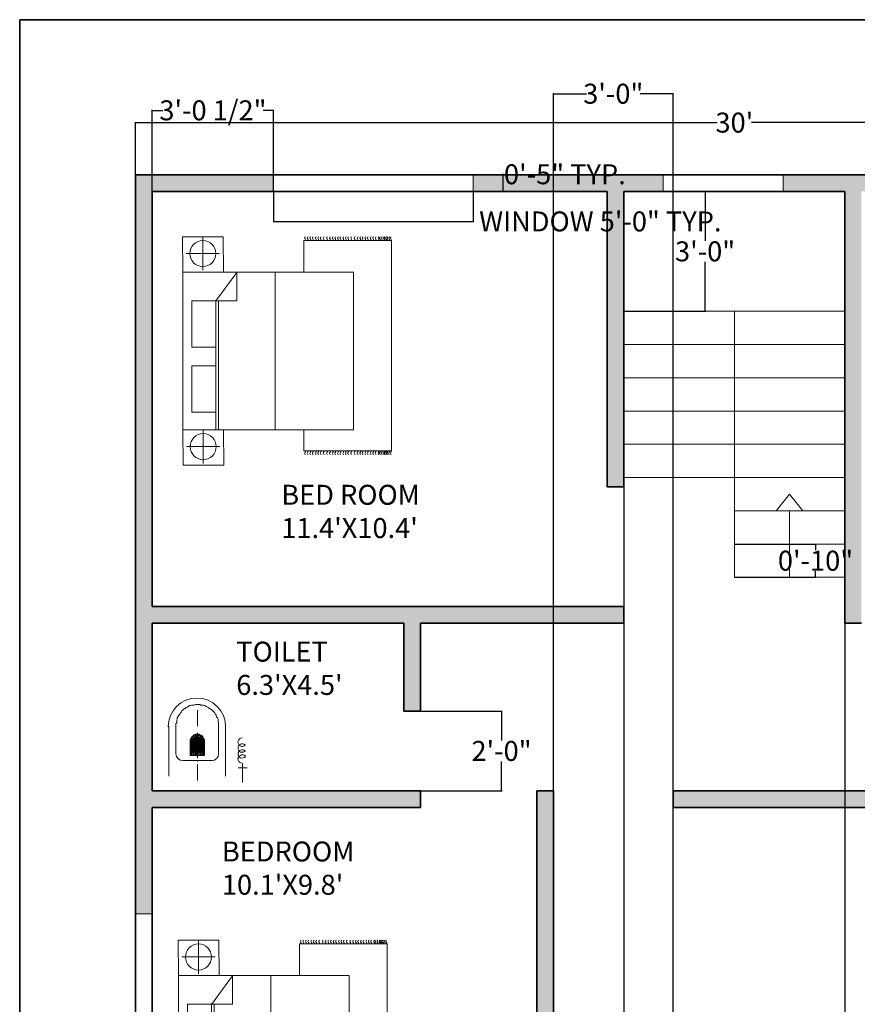
# Model space of a CAD drawing. Units: inches. Extents: x 717 to 1167, y 2046 to 2594.
# Tile 4 of 6: x 720 to 972, y 2298 to 2594. Entities that reach past the tile are written whole.
import ezdxf

# ---------------------------------------------------------------- set-up
doc = ezdxf.new("R2010")
doc.units = ezdxf.units.IN
doc.header["$MEASUREMENT"] = 0
for name, color, linetype, lineweight in [('A-ANNO-DIMS', 2, 'Continuous', 18), ('A-ANNO-SYMB', 7, 'Continuous', 18), ('A-ANNO-TTLB', 7, 'Continuous', 35), ('A-AREA-IDEN', 7, 'Continuous', 18), ('A-FLOR-FIXT', 8, 'Continuous', 18), ('A-FLOR-STRS', 7, 'Continuous', 18), ('A-FURN', 8, 'Continuous', 18), ('A-GLAZ', 4, 'Continuous', 18), ('A-WALL', 7, 'Continuous', 35), ('A-WALL-PATT', 140, 'Continuous', 13)]:
    doc.layers.add(name, color=color, linetype=linetype, lineweight=lineweight)
doc.styles.get("Standard").update_dxf_attribs({"font": 'arial.ttf'})
doc.dimstyles.get("Standard").update_dxf_attribs({"dimtxt": 6, "dimasz": 0.18, "dimexe": 0.18, "dimexo": 0.0625, "dimgap": 0.09, "dimtad": 0, "dimtih": 1, "dimtoh": 1, "dimdec": 1, "dimzin": 0, "dimdsep": 46, "dimlunit": 3, "dimtxsty": 'Standard', "dimcen": 0.09, "dimadec": 0, "dimazin": 0, "dimtfac": 1, "dimtdec": 1, "dimtofl": 0, "dimtmove": 0, "dimatfit": 3, "dimfxl": 1, "dimtolj": 1, "dimtzin": 0, "dimarcsym": 0})

# ---------------------------------------------------------------- blocks, each defined once
blk = doc.blocks.new('*D4')
at = {"layer": 'A-ANNO-DIMS', "color": 0, "lineweight": -2, "transparency": 16777216}
for p, q in [((754.71, 2547.63), (754.71, 2563.46)), ((754.89, 2563.28), (929.54, 2563.28)), ((1114.53, 2563.28), (939.89, 2563.28)), ((1114.71, 2547.63), (1114.71, 2563.46))]:
    blk.add_line(p, q, dxfattribs=at)
at = {"layer": 'A-ANNO-DIMS', "color": 0, "transparency": 16777216}
for points in [[(754.89, 2563.31), (754.89, 2563.25), (754.71, 2563.28)], [(1114.53, 2563.31), (1114.53, 2563.25), (1114.71, 2563.28)]]:
    blk.add_solid(points, dxfattribs=at)
at = {"layer": 'Defpoints', "color": 0, "transparency": 16777216}
for p in [(1114.71, 2563.28), (754.71, 2547.57), (1114.71, 2547.57)]:
    blk.add_point(p, dxfattribs=at)
at = {"layer": 'A-ANNO-DIMS', "color": 0, "transparency": 16777216, "insert": (934.71, 2563.28), "char_height": 6, "attachment_point": 5}
blk.add_mtext("\\A1;30'", dxfattribs=at)
blk = doc.blocks.new('BED-DOUBLE-WITH-NIGHTSTANDS')
for p, q in [((6.09, 68.68), (6.09, 58.62)), ((36.42, 67.59), (62.78, 67.59)), ((36.42, 58.05), (36.42, 67.59)), ((62.78, 67.59), (62.78, 4.35)), ((1.07, 63.65), (11.12, 63.65)), ((9.97, 49.39), (16.32, 58)), ((16.32, 49.44), (16.32, 58)), ((27.82, 58.05), (27.82, 10.63)), ((9.97, 49.44), (16.32, 49.44)), ((9.97, 49.39), (9.97, 10.63)), ((10.78, 49.44), (10.78, 10.63)), ((6.2, 10.63), (6.2, 0.57)), ((36.42, 4.35), (36.42, 10.65)), ((1.17, 5.6), (11.22, 5.6)), ((62.78, 4.35), (36.42, 4.35))]:
    blk.add_line(p, q)
for points in [[(12.29, 58.05), (12.19, 68.68), (0, 68.68), (0.1, 58.05)], [(0.1, 58.05), (51.42, 58.05), (51.42, 10.63), (0.1, 10.63)], [(2.8, 49.44), (9.97, 49.44), (9.97, 35.55), (2.8, 35.55)], [(2.8, 29.88), (9.97, 29.88), (9.97, 15.98), (2.8, 15.98)], [(12.39, 0), (12.29, 10.63), (0.1, 10.63), (0.21, 0)]]:
    blk.add_lwpolyline(points, close=True)
for centre in [(6.09, 63.65), (6.2, 5.6)]:
    blk.add_circle(centre, 3.92)
for points, knots in [([(36.95, 68.71), (36.83, 68.61), (36.59, 68.42), (36.83, 68.08), (37, 67.8), (36.89, 67.65), (36.85, 67.58)], [0, 0, 0, 0, 0.400747, 0.791423, 1.067667, 1.29709, 1.29709, 1.29709, 1.29709]), ([(37.73, 68.71), (37.61, 68.61), (37.37, 68.42), (37.61, 68.08), (37.78, 67.8), (37.67, 67.65), (37.62, 67.58)], [0, 0, 0, 0, 0.400747, 0.791423, 1.067667, 1.29709, 1.29709, 1.29709, 1.29709]), ([(38.54, 68.71), (38.42, 68.61), (38.18, 68.42), (38.42, 68.08), (38.59, 67.8), (38.49, 67.65), (38.44, 67.58)], [0, 0, 0, 0, 0.400747, 0.791423, 1.067667, 1.29709, 1.29709, 1.29709, 1.29709]), ([(39.27, 68.71), (39.15, 68.61), (38.91, 68.42), (39.15, 68.08), (39.32, 67.8), (39.22, 67.65), (39.17, 67.58)], [0, 0, 0, 0, 0.400747, 0.791423, 1.067667, 1.29709, 1.29709, 1.29709, 1.29709]), ([(40.15, 68.71), (40.03, 68.61), (39.79, 68.42), (40.03, 68.08), (40.2, 67.8), (40.1, 67.65), (40.05, 67.58)], [0, 0, 0, 0, 0.400747, 0.791423, 1.067667, 1.29709, 1.29709, 1.29709, 1.29709]), ([(40.91, 68.71), (40.78, 68.61), (40.54, 68.42), (40.78, 68.08), (40.96, 67.8), (40.85, 67.65), (40.8, 67.58)], [0, 0, 0, 0, 0.400747, 0.791423, 1.067667, 1.29709, 1.29709, 1.29709, 1.29709]), ([(41.63, 68.71), (41.51, 68.61), (41.27, 68.42), (41.51, 68.08), (41.69, 67.8), (41.58, 67.65), (41.53, 67.58)], [0, 0, 0, 0, 0.400747, 0.791423, 1.067667, 1.29709, 1.29709, 1.29709, 1.29709]), ([(42.52, 68.71), (42.39, 68.61), (42.16, 68.42), (42.39, 68.08), (42.57, 67.8), (42.46, 67.65), (42.41, 67.58)], [0, 0, 0, 0, 0.400747, 0.791423, 1.067667, 1.29709, 1.29709, 1.29709, 1.29709]), ([(43.55, 68.71), (43.43, 68.61), (43.19, 68.42), (43.43, 68.08), (43.6, 67.8), (43.5, 67.65), (43.45, 67.58)], [0, 0, 0, 0, 0.400747, 0.791423, 1.067667, 1.29709, 1.29709, 1.29709, 1.29709]), ([(44.43, 68.71), (44.31, 68.61), (44.07, 68.42), (44.31, 68.08), (44.49, 67.8), (44.38, 67.65), (44.33, 67.58)], [0, 0, 0, 0, 0.400747, 0.791423, 1.067667, 1.29709, 1.29709, 1.29709, 1.29709]), ([(45.25, 68.71), (45.13, 68.61), (44.89, 68.42), (45.13, 68.08), (45.3, 67.8), (45.2, 67.65), (45.15, 67.58)], [0, 0, 0, 0, 0.400747, 0.791423, 1.067667, 1.29709, 1.29709, 1.29709, 1.29709]), ([(46.03, 68.71), (45.91, 68.61), (45.67, 68.42), (45.91, 68.08), (46.08, 67.8), (45.97, 67.65), (45.92, 67.58)], [0, 0, 0, 0, 0.400747, 0.791423, 1.067667, 1.29709, 1.29709, 1.29709, 1.29709]), ([(46.84, 68.71), (46.72, 68.61), (46.48, 68.42), (46.72, 68.08), (46.9, 67.8), (46.79, 67.65), (46.74, 67.58)], [0, 0, 0, 0, 0.400747, 0.791423, 1.067667, 1.29709, 1.29709, 1.29709, 1.29709]), ([(47.57, 68.71), (47.45, 68.61), (47.21, 68.42), (47.45, 68.08), (47.62, 67.8), (47.52, 67.65), (47.47, 67.58)], [0, 0, 0, 0, 0.400747, 0.791423, 1.067667, 1.29709, 1.29709, 1.29709, 1.29709]), ([(48.45, 68.71), (48.33, 68.61), (48.09, 68.42), (48.33, 68.08), (48.51, 67.8), (48.4, 67.65), (48.35, 67.58)], [0, 0, 0, 0, 0.400747, 0.791423, 1.067667, 1.29709, 1.29709, 1.29709, 1.29709]), ([(49.21, 68.71), (49.08, 68.61), (48.85, 68.42), (49.08, 68.08), (49.26, 67.8), (49.15, 67.65), (49.1, 67.58)], [0, 0, 0, 0, 0.400747, 0.791423, 1.067667, 1.29709, 1.29709, 1.29709, 1.29709]), ([(49.93, 68.71), (49.81, 68.61), (49.57, 68.42), (49.81, 68.08), (49.99, 67.8), (49.88, 67.65), (49.83, 67.58)], [0, 0, 0, 0, 0.400747, 0.791423, 1.067667, 1.29709, 1.29709, 1.29709, 1.29709]), ([(50.82, 68.71), (50.69, 68.61), (50.46, 68.42), (50.69, 68.08), (50.87, 67.8), (50.76, 67.65), (50.71, 67.58)], [0, 0, 0, 0, 0.400747, 0.791423, 1.067667, 1.29709, 1.29709, 1.29709, 1.29709]), ([(51.85, 68.71), (51.73, 68.61), (51.49, 68.42), (51.73, 68.08), (51.9, 67.8), (51.8, 67.65), (51.75, 67.58)], [0, 0, 0, 0, 0.400747, 0.791423, 1.067667, 1.29709, 1.29709, 1.29709, 1.29709]), ([(52.74, 68.71), (52.61, 68.61), (52.37, 68.42), (52.61, 68.08), (52.79, 67.8), (52.68, 67.65), (52.63, 67.58)], [0, 0, 0, 0, 0.400747, 0.791423, 1.067667, 1.29709, 1.29709, 1.29709, 1.29709]), ([(53.55, 68.71), (53.43, 68.61), (53.19, 68.42), (53.43, 68.08), (53.6, 67.8), (53.5, 67.65), (53.45, 67.58)], [0, 0, 0, 0, 0.400747, 0.791423, 1.067667, 1.29709, 1.29709, 1.29709, 1.29709]), ([(54.24, 68.71), (54.12, 68.61), (53.88, 68.42), (54.12, 68.08), (54.29, 67.8), (54.19, 67.65), (54.14, 67.58)], [0, 0, 0, 0, 0.400747, 0.791423, 1.067667, 1.29709, 1.29709, 1.29709, 1.29709]), ([(55.06, 68.71), (54.94, 68.61), (54.7, 68.42), (54.94, 68.08), (55.11, 67.8), (55, 67.65), (54.95, 67.58)], [0, 0, 0, 0, 0.400747, 0.791423, 1.067667, 1.29709, 1.29709, 1.29709, 1.29709]), ([(55.78, 68.71), (55.66, 68.61), (55.42, 68.42), (55.66, 68.08), (55.84, 67.8), (55.73, 67.65), (55.68, 67.58)], [0, 0, 0, 0, 0.400747, 0.791423, 1.067667, 1.29709, 1.29709, 1.29709, 1.29709]), ([(56.67, 68.71), (56.55, 68.61), (56.31, 68.42), (56.55, 68.08), (56.72, 67.8), (56.61, 67.65), (56.56, 67.58)], [0, 0, 0, 0, 0.400747, 0.791423, 1.067667, 1.29709, 1.29709, 1.29709, 1.29709]), ([(57.42, 68.71), (57.3, 68.61), (57.06, 68.42), (57.3, 68.08), (57.47, 67.8), (57.36, 67.65), (57.32, 67.58)], [0, 0, 0, 0, 0.400747, 0.791423, 1.067667, 1.29709, 1.29709, 1.29709, 1.29709]), ([(58.15, 68.71), (58.03, 68.61), (57.79, 68.42), (58.03, 68.08), (58.2, 67.8), (58.1, 67.66), (58.05, 67.59)], [0, 0, 0, 0, 0.400747, 0.791423, 1.067667, 1.283686, 1.283686, 1.283686, 1.283686]), ([(59.03, 68.71), (58.91, 68.61), (58.67, 68.42), (58.91, 68.08), (59.08, 67.8), (58.98, 67.66), (58.93, 67.59)], [0, 0, 0, 0, 0.400747, 0.791423, 1.067667, 1.283686, 1.283686, 1.283686, 1.283686]), ([(59.46, 68.71), (59.34, 68.61), (59.09, 68.42), (59.34, 68.08), (59.51, 67.8), (59.41, 67.66), (59.36, 67.59)], [0, 0, 0, 0, 0.402903, 0.794912, 1.071156, 1.287177, 1.287177, 1.287177, 1.287177]), ([(60.05, 68.71), (59.93, 68.61), (59.69, 68.42), (59.93, 68.08), (60.1, 67.8), (60, 67.66), (59.96, 67.59)], [0, 0, 0, 0, 0.400747, 0.791423, 1.067667, 1.283686, 1.283686, 1.283686, 1.283686]), ([(60.63, 68.71), (60.51, 68.61), (60.27, 68.42), (60.51, 68.08), (60.68, 67.8), (60.58, 67.66), (60.53, 67.59)], [0, 0, 0, 0, 0.400747, 0.791423, 1.067667, 1.283686, 1.283686, 1.283686, 1.283686]), ([(60.94, 68.71), (60.82, 68.61), (60.58, 68.42), (60.81, 68.08), (60.99, 67.8), (60.89, 67.66), (60.84, 67.59)], [0, 0, 0, 0, 0.400747, 0.791423, 1.067667, 1.283686, 1.283686, 1.283686, 1.283686]), ([(61.36, 68.71), (61.23, 68.61), (60.99, 68.42), (61.23, 68.08), (61.41, 67.8), (61.3, 67.65), (61.25, 67.58)], [0, 0, 0, 0, 0.400747, 0.791423, 1.067667, 1.29709, 1.29709, 1.29709, 1.29709]), ([(61.75, 68.71), (61.63, 68.61), (61.39, 68.42), (61.63, 68.08), (61.8, 67.8), (61.7, 67.65), (61.65, 67.58)], [0, 0, 0, 0, 0.400747, 0.791423, 1.067667, 1.29709, 1.29709, 1.29709, 1.29709]), ([(62.24, 68.71), (62.12, 68.61), (61.88, 68.42), (62.12, 68.08), (62.29, 67.8), (62.18, 67.65), (62.13, 67.58)], [0, 0, 0, 0, 0.400747, 0.791423, 1.067667, 1.29709, 1.29709, 1.29709, 1.29709]), ([(62.71, 68.71), (62.59, 68.61), (62.35, 68.42), (62.59, 68.08), (62.76, 67.8), (62.66, 67.65), (62.61, 67.58)], [0, 0, 0, 0, 0.400747, 0.791423, 1.067667, 1.29709, 1.29709, 1.29709, 1.29709]), ([(36.95, 3.23), (36.83, 3.32), (36.59, 3.52), (36.83, 3.86), (37, 4.14), (36.89, 4.29), (36.85, 4.35)], [0, 0, 0, 0, 0.400747, 0.791423, 1.067667, 1.29709, 1.29709, 1.29709, 1.29709]), ([(37.73, 3.23), (37.61, 3.32), (37.37, 3.52), (37.61, 3.86), (37.78, 4.14), (37.67, 4.29), (37.62, 4.35)], [0, 0, 0, 0, 0.400747, 0.791423, 1.067667, 1.29709, 1.29709, 1.29709, 1.29709]), ([(38.54, 3.23), (38.42, 3.32), (38.18, 3.52), (38.42, 3.86), (38.59, 4.14), (38.49, 4.29), (38.44, 4.35)], [0, 0, 0, 0, 0.400747, 0.791423, 1.067667, 1.29709, 1.29709, 1.29709, 1.29709]), ([(39.27, 3.23), (39.15, 3.32), (38.91, 3.52), (39.15, 3.86), (39.32, 4.14), (39.22, 4.29), (39.17, 4.35)], [0, 0, 0, 0, 0.400747, 0.791423, 1.067667, 1.29709, 1.29709, 1.29709, 1.29709]), ([(40.15, 3.23), (40.03, 3.32), (39.79, 3.52), (40.03, 3.86), (40.2, 4.14), (40.1, 4.29), (40.05, 4.35)], [0, 0, 0, 0, 0.400747, 0.791423, 1.067667, 1.29709, 1.29709, 1.29709, 1.29709]), ([(40.91, 3.23), (40.78, 3.32), (40.54, 3.52), (40.78, 3.86), (40.96, 4.14), (40.85, 4.29), (40.8, 4.35)], [0, 0, 0, 0, 0.400747, 0.791423, 1.067667, 1.29709, 1.29709, 1.29709, 1.29709]), ([(41.63, 3.23), (41.51, 3.32), (41.27, 3.52), (41.51, 3.86), (41.69, 4.14), (41.58, 4.29), (41.53, 4.35)], [0, 0, 0, 0, 0.400747, 0.791423, 1.067667, 1.29709, 1.29709, 1.29709, 1.29709]), ([(42.52, 3.23), (42.39, 3.32), (42.16, 3.52), (42.39, 3.86), (42.57, 4.14), (42.46, 4.29), (42.41, 4.35)], [0, 0, 0, 0, 0.400747, 0.791423, 1.067667, 1.29709, 1.29709, 1.29709, 1.29709]), ([(43.55, 3.23), (43.43, 3.32), (43.19, 3.52), (43.43, 3.86), (43.6, 4.14), (43.5, 4.29), (43.45, 4.35)], [0, 0, 0, 0, 0.400747, 0.791423, 1.067667, 1.29709, 1.29709, 1.29709, 1.29709]), ([(44.43, 3.23), (44.31, 3.32), (44.07, 3.52), (44.31, 3.86), (44.49, 4.14), (44.38, 4.29), (44.33, 4.35)], [0, 0, 0, 0, 0.400747, 0.791423, 1.067667, 1.29709, 1.29709, 1.29709, 1.29709]), ([(45.25, 3.23), (45.13, 3.32), (44.89, 3.52), (45.13, 3.86), (45.3, 4.14), (45.2, 4.29), (45.15, 4.35)], [0, 0, 0, 0, 0.400747, 0.791423, 1.067667, 1.29709, 1.29709, 1.29709, 1.29709]), ([(46.03, 3.23), (45.91, 3.32), (45.67, 3.52), (45.91, 3.86), (46.08, 4.14), (45.97, 4.29), (45.92, 4.35)], [0, 0, 0, 0, 0.400747, 0.791423, 1.067667, 1.29709, 1.29709, 1.29709, 1.29709]), ([(46.84, 3.23), (46.72, 3.32), (46.48, 3.52), (46.72, 3.86), (46.9, 4.14), (46.79, 4.29), (46.74, 4.35)], [0, 0, 0, 0, 0.400747, 0.791423, 1.067667, 1.29709, 1.29709, 1.29709, 1.29709]), ([(47.57, 3.23), (47.45, 3.32), (47.21, 3.52), (47.45, 3.86), (47.62, 4.14), (47.52, 4.29), (47.47, 4.35)], [0, 0, 0, 0, 0.400747, 0.791423, 1.067667, 1.29709, 1.29709, 1.29709, 1.29709]), ([(48.45, 3.23), (48.33, 3.32), (48.09, 3.52), (48.33, 3.86), (48.51, 4.14), (48.4, 4.29), (48.35, 4.35)], [0, 0, 0, 0, 0.400747, 0.791423, 1.067667, 1.29709, 1.29709, 1.29709, 1.29709]), ([(49.21, 3.23), (49.08, 3.32), (48.85, 3.52), (49.08, 3.86), (49.26, 4.14), (49.15, 4.29), (49.1, 4.35)], [0, 0, 0, 0, 0.400747, 0.791423, 1.067667, 1.29709, 1.29709, 1.29709, 1.29709]), ([(49.93, 3.23), (49.81, 3.32), (49.57, 3.52), (49.81, 3.86), (49.99, 4.14), (49.88, 4.29), (49.83, 4.35)], [0, 0, 0, 0, 0.400747, 0.791423, 1.067667, 1.29709, 1.29709, 1.29709, 1.29709]), ([(50.82, 3.23), (50.69, 3.32), (50.46, 3.52), (50.69, 3.86), (50.87, 4.14), (50.76, 4.29), (50.71, 4.35)], [0, 0, 0, 0, 0.400747, 0.791423, 1.067667, 1.29709, 1.29709, 1.29709, 1.29709]), ([(51.85, 3.23), (51.73, 3.32), (51.49, 3.52), (51.73, 3.86), (51.9, 4.14), (51.8, 4.29), (51.75, 4.35)], [0, 0, 0, 0, 0.400747, 0.791423, 1.067667, 1.29709, 1.29709, 1.29709, 1.29709]), ([(52.74, 3.23), (52.61, 3.32), (52.37, 3.52), (52.61, 3.86), (52.79, 4.14), (52.68, 4.29), (52.63, 4.35)], [0, 0, 0, 0, 0.400747, 0.791423, 1.067667, 1.29709, 1.29709, 1.29709, 1.29709]), ([(53.55, 3.23), (53.43, 3.32), (53.19, 3.52), (53.43, 3.86), (53.6, 4.14), (53.5, 4.29), (53.45, 4.35)], [0, 0, 0, 0, 0.400747, 0.791423, 1.067667, 1.29709, 1.29709, 1.29709, 1.29709]), ([(54.24, 3.23), (54.12, 3.32), (53.88, 3.52), (54.12, 3.86), (54.29, 4.14), (54.19, 4.29), (54.14, 4.35)], [0, 0, 0, 0, 0.400747, 0.791423, 1.067667, 1.29709, 1.29709, 1.29709, 1.29709]), ([(55.06, 3.23), (54.94, 3.32), (54.7, 3.52), (54.94, 3.86), (55.11, 4.14), (55, 4.29), (54.95, 4.35)], [0, 0, 0, 0, 0.400747, 0.791423, 1.067667, 1.29709, 1.29709, 1.29709, 1.29709]), ([(55.78, 3.23), (55.66, 3.32), (55.42, 3.52), (55.66, 3.86), (55.84, 4.14), (55.73, 4.29), (55.68, 4.35)], [0, 0, 0, 0, 0.400747, 0.791423, 1.067667, 1.29709, 1.29709, 1.29709, 1.29709]), ([(56.67, 3.23), (56.55, 3.32), (56.31, 3.52), (56.55, 3.86), (56.72, 4.14), (56.61, 4.29), (56.56, 4.35)], [0, 0, 0, 0, 0.400747, 0.791423, 1.067667, 1.29709, 1.29709, 1.29709, 1.29709]), ([(57.42, 3.23), (57.3, 3.32), (57.06, 3.52), (57.3, 3.86), (57.47, 4.14), (57.36, 4.29), (57.32, 4.35)], [0, 0, 0, 0, 0.400747, 0.791423, 1.067667, 1.29709, 1.29709, 1.29709, 1.29709]), ([(58.15, 3.23), (58.03, 3.32), (57.79, 3.52), (58.03, 3.86), (58.2, 4.14), (58.09, 4.29), (58.04, 4.35)], [0, 0, 0, 0, 0.400747, 0.791423, 1.067667, 1.29709, 1.29709, 1.29709, 1.29709]), ([(59.03, 3.23), (58.91, 3.32), (58.67, 3.52), (58.91, 3.86), (59.08, 4.14), (58.98, 4.29), (58.93, 4.35)], [0, 0, 0, 0, 0.400747, 0.791423, 1.067667, 1.29709, 1.29709, 1.29709, 1.29709]), ([(59.46, 3.23), (59.33, 3.32), (59.08, 3.51), (59.34, 3.86), (59.51, 4.14), (59.4, 4.29), (59.36, 4.35)], [0, 0, 0, 0, 0.407265, 0.802015, 1.07826, 1.307683, 1.307683, 1.307683, 1.307683]), ([(60.03, 3.23), (59.9, 3.32), (59.67, 3.52), (59.9, 3.86), (60.08, 4.14), (59.97, 4.29), (59.92, 4.35)], [0, 0, 0, 0, 0.400747, 0.791423, 1.067667, 1.29709, 1.29709, 1.29709, 1.29709]), ([(60.6, 3.23), (60.48, 3.32), (60.24, 3.52), (60.48, 3.86), (60.65, 4.14), (60.54, 4.29), (60.5, 4.35)], [0, 0, 0, 0, 0.400747, 0.791423, 1.067667, 1.29709, 1.29709, 1.29709, 1.29709]), ([(60.91, 3.23), (60.79, 3.32), (60.55, 3.52), (60.79, 3.86), (60.96, 4.14), (60.85, 4.29), (60.81, 4.35)], [0, 0, 0, 0, 0.400747, 0.791423, 1.067667, 1.29709, 1.29709, 1.29709, 1.29709]), ([(61.33, 3.23), (61.21, 3.32), (60.97, 3.52), (61.21, 3.86), (61.38, 4.14), (61.27, 4.29), (61.22, 4.35)], [0, 0, 0, 0, 0.400747, 0.791423, 1.067667, 1.29709, 1.29709, 1.29709, 1.29709]), ([(61.72, 3.23), (61.6, 3.32), (61.36, 3.52), (61.6, 3.86), (61.78, 4.14), (61.67, 4.29), (61.62, 4.35)], [0, 0, 0, 0, 0.400747, 0.791423, 1.067667, 1.29709, 1.29709, 1.29709, 1.29709]), ([(62.21, 3.23), (62.09, 3.32), (61.85, 3.52), (62.09, 3.86), (62.26, 4.14), (62.15, 4.29), (62.11, 4.35)], [0, 0, 0, 0, 0.400747, 0.791423, 1.067667, 1.29709, 1.29709, 1.29709, 1.29709]), ([(62.71, 3.23), (62.59, 3.32), (62.35, 3.52), (62.59, 3.86), (62.76, 4.14), (62.66, 4.29), (62.61, 4.35)], [0, 0, 0, 0, 0.400747, 0.791423, 1.067667, 1.29709, 1.29709, 1.29709, 1.29709])]:
    blk.add_open_spline(points, degree=3, knots=knots)
blk = doc.blocks.new('WC-PLAN')
h = blk.add_hatch(color=256)
h.paths.add_polyline_path([(6.83, 8.12), (6.83, 13.2), (6.6, 8.12)])
h.paths.add_polyline_path([(6.83, 13.2), (6.6, 8.12), (6.6, 12.82)])
h.paths.add_polyline_path([(6.6, 8.12), (6.6, 12.82), (6.6, 12.44)])
h = blk.add_hatch(color=256)
h.paths.add_polyline_path([(7.05, 8.12), (7.05, 13.58), (6.83, 8.12)])
h.paths.add_polyline_path([(7.05, 13.58), (6.83, 8.12), (6.83, 13.2)])
h = blk.add_hatch(color=256)
h.paths.add_polyline_path([(7.21, 8.12), (7.21, 13.81), (7.05, 8.12)])
h.paths.add_polyline_path([(7.21, 13.81), (7.05, 8.12), (7.05, 13.58)])
h = blk.add_hatch(color=256)
h.paths.add_polyline_path([(7.59, 8.12), (7.59, 14.19), (7.21, 8.12)])
h.paths.add_polyline_path([(7.59, 14.19), (7.21, 8.12), (7.21, 13.81)])
h = blk.add_hatch(color=256)
h.paths.add_polyline_path([(7.81, 8.12), (7.81, 14.34), (7.59, 8.12)])
h.paths.add_polyline_path([(7.81, 14.34), (7.59, 8.12), (7.59, 14.19)])
h = blk.add_hatch(color=256)
h.paths.add_polyline_path([(8.19, 8.12), (8.19, 14.56), (7.81, 8.12)])
h.paths.add_polyline_path([(8.19, 14.56), (7.81, 8.12), (7.81, 14.34)])
h = blk.add_hatch(color=256)
h.paths.add_polyline_path([(8.57, 8.12), (8.57, 14.56), (8.19, 8.12)])
h.paths.add_polyline_path([(8.57, 14.56), (8.19, 8.12), (8.19, 14.56)])
h = blk.add_hatch(color=256)
h.paths.add_polyline_path([(8.95, 8.12), (8.95, 14.56), (8.57, 8.12)])
h.paths.add_polyline_path([(8.95, 14.56), (8.57, 8.12), (8.57, 14.56)])
h = blk.add_hatch(color=256)
h.paths.add_polyline_path([(9.33, 8.12), (9.33, 14.56), (8.95, 8.12)])
h.paths.add_polyline_path([(9.33, 14.56), (8.95, 8.12), (8.95, 14.56)])
h = blk.add_hatch(color=256)
h.paths.add_polyline_path([(9.71, 8.12), (9.71, 14.34), (9.33, 8.12)])
h.paths.add_polyline_path([(9.71, 14.34), (9.33, 8.12), (9.33, 14.56)])
h = blk.add_hatch(color=256)
h.paths.add_polyline_path([(10.16, 8.12), (10.16, 14.19), (9.71, 8.12)])
h.paths.add_polyline_path([(10.16, 14.19), (9.71, 8.12), (9.71, 14.34)])
h = blk.add_hatch(color=256)
h.paths.add_polyline_path([(10.32, 8.12), (10.32, 13.81), (10.16, 8.12)])
h.paths.add_polyline_path([(10.32, 13.81), (10.16, 8.12), (10.16, 14.19)])
h = blk.add_hatch(color=256)
h.paths.add_polyline_path([(10.54, 8.12), (10.54, 13.58), (10.32, 8.12)])
h.paths.add_polyline_path([(10.54, 13.58), (10.32, 8.12), (10.32, 13.81)])
h = blk.add_hatch(color=256)
h.paths.add_polyline_path([(10.7, 8.12), (10.7, 13.2), (10.54, 8.12)])
h.paths.add_polyline_path([(10.7, 13.2), (10.54, 8.12), (10.54, 13.58)])
h = blk.add_hatch(color=256)
h.paths.add_polyline_path([(10.92, 8.12), (10.92, 12.82), (10.7, 8.12)])
h.paths.add_polyline_path([(10.92, 12.82), (10.7, 8.12), (10.7, 13.2)])
for points in [[(2.35, 15.93), (2.35, 16.69), (2.35, 17.3), (2.35, 17.67), (2.58, 18.05), (2.58, 18.43), (2.58, 18.66), (2.73, 19.04), (2.73, 19.42), (2.96, 19.8), (3.11, 20.03), (3.34, 20.41), (3.49, 20.56), (3.72, 20.94), (3.94, 21.16), (4.1, 21.54), (4.32, 21.77), (4.48, 21.92), (4.85, 22.15), (5.08, 22.3), (5.46, 22.53), (5.69, 22.68), (6.07, 22.91), (6.45, 23.14), (6.6, 23.14), (7.05, 23.29), (7.43, 23.29), (7.81, 23.29), (8.19, 23.52), (8.8, 23.52), (9.56, 23.52), (9.71, 23.29), (10.16, 23.29), (10.54, 23.29), (10.92, 23.14), (11.07, 23.14), (11.45, 22.91), (11.91, 22.68), (12.06, 22.53), (12.44, 22.3), (12.67, 22.15), (13.05, 21.92), (13.2, 21.77), (13.43, 21.54), (13.81, 21.16), (14.03, 20.94), (14.18, 20.56), (14.41, 20.41), (14.41, 20.03), (14.56, 19.8), (14.79, 19.42), (15.02, 19.04), (15.02, 18.66), (15.02, 18.43), (15.17, 18.05), (15.17, 17.67), (15.17, 17.3), (15.17, 16.69), (15.17, 15.93)], [(8.8, 16.92), (8.8, 21.77), (8.8, 21.77)], [(0.23, 1.9), (0.23, 16.92), (0.23, 16.92)], [(2.35, 8.72), (2.35, 15.93), (2.35, 15.93)], [(8.8, 7.36), (8.8, 14.94), (8.8, 14.94)], [(15.17, 8.72), (15.17, 15.93), (15.17, 15.93)], [(17.29, 1.9), (17.29, 16.92), (17.29, 16.92)], [(6.6, 8.12), (6.6, 12.44), (6.6, 12.44)], [(10.92, 8.12), (10.92, 12.44), (10.92, 12.44)], [(4.48, 6.6), (13.2, 6.6), (13.2, 6.6)], [(6.6, 8.12), (10.92, 8.12), (10.92, 8.12)], [(8.34, 8.57), (8.57, 8.57), (8.8, 8.57)], [(8.34, 8.57), (8.34, 8.5), (8.34, 8.5)], [(8.8, 8.57), (8.72, 8.5), (8.72, 8.5)], [(8.8, 6.37), (8.72, 6.37), (8.72, 6.37)], [(8.8, 8.57), (8.95, 8.57), (9.18, 8.57)], [(9.18, 8.57), (9.18, 8.5), (9.18, 8.5)], [(8.8, 0.61), (8.8, 5.46), (8.8, 5.46)], [(21.03, 4.48), (23.77, 4.48), (23.77, 4.48)], [(22.4, 0), (22.4, 5.84), (22.4, 5.84)]]:
    blk.add_lwpolyline(points)
for points in [[(6.83, 8.12), (6.83, 13.2), (6.6, 8.12)], [(6.83, 13.2), (6.6, 8.12), (6.6, 12.82)], [(6.6, 8.12), (6.6, 12.82), (6.6, 12.44)], [(6.6, 12.82), (6.6, 8.12), (6.6, 8.12)], [(7.05, 8.12), (7.05, 13.58), (6.83, 8.12)], [(7.05, 13.58), (6.83, 8.12), (6.83, 13.2)], [(7.21, 8.12), (7.21, 13.81), (7.05, 8.12)], [(7.21, 13.81), (7.05, 8.12), (7.05, 13.58)], [(7.59, 8.12), (7.59, 14.19), (7.21, 8.12)], [(7.59, 14.19), (7.21, 8.12), (7.21, 13.81)], [(7.81, 8.12), (7.81, 14.34), (7.59, 8.12)], [(7.81, 14.34), (7.59, 8.12), (7.59, 14.19)], [(8.19, 8.12), (8.19, 14.56), (7.81, 8.12)], [(8.19, 14.56), (7.81, 8.12), (7.81, 14.34)], [(8.57, 8.12), (8.57, 14.56), (8.19, 8.12)], [(8.57, 14.56), (8.19, 8.12), (8.19, 14.56)], [(8.95, 8.12), (8.95, 14.56), (8.57, 8.12)], [(8.95, 14.56), (8.57, 8.12), (8.57, 14.56)], [(9.33, 8.12), (9.33, 14.56), (8.95, 8.12)], [(9.33, 14.56), (8.95, 8.12), (8.95, 14.56)], [(9.71, 14.34), (9.33, 8.12), (9.33, 14.56)], [(9.71, 8.12), (9.71, 14.34), (9.33, 8.12)], [(10.16, 14.19), (9.71, 8.12), (9.71, 14.34)], [(10.16, 8.12), (10.16, 14.19), (9.71, 8.12)], [(10.32, 13.81), (10.16, 8.12), (10.16, 14.19)], [(10.32, 8.12), (10.32, 13.81), (10.16, 8.12)], [(10.54, 13.58), (10.32, 8.12), (10.32, 13.81)], [(10.54, 8.12), (10.54, 13.58), (10.32, 8.12)], [(10.7, 13.2), (10.54, 8.12), (10.54, 13.58)], [(10.7, 8.12), (10.7, 13.2), (10.54, 8.12)], [(10.92, 12.82), (10.7, 8.12), (10.7, 13.2)], [(10.92, 8.12), (10.92, 12.82), (10.7, 8.12)], [(10.92, 12.44), (10.92, 8.12), (10.92, 12.82)], [(10.92, 8.12), (10.92, 12.44)]]:
    blk.add_lwpolyline(points, close=True)
for points, knots in [([(17.29, 16.76), (17.29, 21.54), (13.43, 25.41), (8.65, 25.41), (8.65, 25.41), (3.87, 25.41), (0, 21.54), (0, 16.76)], [0, 0, 0, 0, 0.125, 0.125, 0.125, 0.125001, 1, 1, 1, 1]), ([(10.7, 12.29), (10.7, 13.43), (9.79, 14.34), (8.65, 14.34), (8.65, 14.34), (7.51, 14.34), (6.6, 13.43), (6.6, 12.29)], [0, 0, 0, 0, 0.125, 0.125, 0.125, 0.125001, 1, 1, 1, 1]), ([(22.25, 13.43), (21.72, 13.43), (21.19, 12.97), (21.03, 12.44), (21.03, 12.44), (20.88, 11.91), (21.19, 11.3), (21.64, 11), (21.64, 11), (22.17, 10.77), (22.78, 10.85), (23.16, 11.23)], [0, 0, 0, 0, 0.083333, 0.083333, 0.083333, 0.083334, 0.166667, 0.166667, 0.166667, 0.166668, 1, 1, 1, 1]), ([(23.23, 11.23), (22.86, 11.61), (22.32, 11.76), (21.79, 11.53), (21.79, 11.53), (21.34, 11.38), (21.03, 10.92), (21.03, 10.39), (21.03, 10.39), (21.03, 9.86), (21.34, 9.41), (21.79, 9.18), (21.79, 9.18), (22.32, 9.03), (22.86, 9.18), (23.23, 9.56)], [0, 0, 0, 0, 0.0625, 0.0625, 0.0625, 0.062501, 0.125, 0.125, 0.125, 0.125001, 0.1875, 0.1875, 0.1875, 0.187501, 1, 1, 1, 1]), ([(23.16, 9.48), (22.86, 9.86), (22.25, 10.01), (21.79, 9.79), (21.79, 9.79), (21.34, 9.63), (21.03, 9.1), (21.03, 8.65), (21.03, 8.65), (21.03, 8.12), (21.34, 7.66), (21.79, 7.43), (21.79, 7.43), (22.32, 7.28), (22.86, 7.43), (23.23, 7.81)], [0, 0, 0, 0, 0.0625, 0.0625, 0.0625, 0.062501, 0.125, 0.125, 0.125, 0.125001, 0.1875, 0.1875, 0.1875, 0.187501, 1, 1, 1, 1]), ([(23.23, 7.96), (22.86, 8.34), (22.17, 8.5), (21.72, 8.19), (21.72, 8.19), (21.19, 7.89), (20.88, 7.36), (21.03, 6.75), (21.03, 6.75), (21.19, 6.22), (21.72, 5.84), (22.25, 5.84)], [0, 0, 0, 0, 0.083333, 0.083333, 0.083333, 0.083334, 0.166667, 0.166667, 0.166667, 0.166668, 1, 1, 1, 1])]:
    blk.add_open_spline(points, degree=3, knots=knots)
for points in [[(2.35, 8.65), (2.35, 7.51), (3.26, 6.6), (4.4, 6.6)], [(13.12, 6.6), (14.26, 6.6), (15.17, 7.51), (15.17, 8.65)]]:
    blk.add_open_spline(points, degree=3)
blk = doc.blocks.new('WINDOW-60IN')
for p, q in [((0, 5), (0, 0)), ((60, 5), (0, 5)), ((60, 0), (60, 5)), ((0, 0), (60, 0))]:
    blk.add_line(p, q)
blk = doc.blocks.new('*D13')
at = {"layer": 'A-ANNO-DIMS', "color": 0, "lineweight": -2, "transparency": 16777216}
for p, q in [((796.2, 2542.51), (796.2, 2533.39)), ((856.2, 2542.51), (856.2, 2533.39)), ((796.38, 2533.57), (856.02, 2533.57)), ((856.2, 2533.57), (856.38, 2533.57))]:
    blk.add_line(p, q, dxfattribs=at)
at = {"layer": 'A-ANNO-DIMS', "color": 0, "transparency": 16777216}
for points in [[(796.38, 2533.6), (796.38, 2533.54), (796.2, 2533.57)], [(856.02, 2533.6), (856.02, 2533.54), (856.2, 2533.57)]]:
    blk.add_solid(points, dxfattribs=at)
at = {"layer": 'Defpoints', "color": 0, "transparency": 16777216}
for p in [(796.2, 2542.57), (856.2, 2542.57), (856.2, 2533.57)]:
    blk.add_point(p, dxfattribs=at)
at = {"layer": 'A-ANNO-DIMS', "color": 0, "transparency": 16777216, "insert": (894.43, 2533.57), "char_height": 6, "attachment_point": 5}
blk.add_mtext('\\A1;WINDOW 5\'-0" TYP.', dxfattribs=at)
blk = doc.blocks.new('*D14')
at = {"layer": 'A-ANNO-DIMS', "color": 0, "lineweight": -2, "transparency": 16777216}
for p, q in [((856.26, 2547.57), (865.38, 2547.57)), ((865.2, 2547.57), (865.2, 2547.75)), ((865.2, 2547.75), (865.38, 2547.75)), ((865.2, 2542.75), (865.2, 2547.39)), ((856.26, 2542.57), (865.38, 2542.57))]:
    blk.add_line(p, q, dxfattribs=at)
at = {"layer": 'A-ANNO-DIMS', "color": 0, "transparency": 16777216}
for points in [[(865.17, 2547.39), (865.23, 2547.39), (865.2, 2547.57)], [(865.17, 2542.75), (865.23, 2542.75), (865.2, 2542.57)]]:
    blk.add_solid(points, dxfattribs=at)
at = {"layer": 'Defpoints', "color": 0, "transparency": 16777216}
for p in [(856.2, 2547.57), (865.2, 2547.57), (856.2, 2542.57)]:
    blk.add_point(p, dxfattribs=at)
at = {"layer": 'A-ANNO-DIMS', "color": 0, "transparency": 16777216, "insert": (883.76, 2547.75), "char_height": 6, "attachment_point": 5}
blk.add_mtext('\\A1;0\'-5" TYP.', dxfattribs=at)
blk = doc.blocks.new('*D35')
at = {"layer": 'A-ANNO-DIMS', "color": 0, "lineweight": -2, "transparency": 16777216}
for p, q in [((901.51, 2542.51), (901.51, 2054.99)), ((967.91, 2542.51), (967.91, 2054.99)), ((901.69, 2055.17), (919.66, 2055.17)), ((967.73, 2055.17), (949.77, 2055.17))]:
    blk.add_line(p, q, dxfattribs=at)
at = {"layer": 'A-ANNO-DIMS', "color": 0, "transparency": 16777216}
for points in [[(901.69, 2055.2), (901.69, 2055.14), (901.51, 2055.17)], [(967.73, 2055.2), (967.73, 2055.14), (967.91, 2055.17)]]:
    blk.add_solid(points, dxfattribs=at)
at = {"layer": 'Defpoints', "color": 0, "transparency": 16777216}
for p in [(901.51, 2542.57), (967.91, 2542.57), (967.91, 2055.17)]:
    blk.add_point(p, dxfattribs=at)
at = {"layer": 'A-ANNO-DIMS', "color": 0, "transparency": 16777216, "insert": (934.71, 2055.17), "char_height": 6, "attachment_point": 5}
blk.add_mtext('\\A1;5\'-6 1/2"', dxfattribs=at)
blk = doc.blocks.new('*D38')
at = {"layer": 'A-ANNO-DIMS', "color": 0, "lineweight": -2, "transparency": 16777216}
for p, q in [((880.31, 2079.63), (880.31, 2572.15)), ((880.49, 2571.97), (890.25, 2571.97)), ((916.13, 2571.97), (906.38, 2571.97)), ((916.31, 2122.83), (916.31, 2572.15))]:
    blk.add_line(p, q, dxfattribs=at)
at = {"layer": 'A-ANNO-DIMS', "color": 0, "transparency": 16777216}
for points in [[(880.49, 2572), (880.49, 2571.94), (880.31, 2571.97)], [(916.13, 2572), (916.13, 2571.94), (916.31, 2571.97)]]:
    blk.add_solid(points, dxfattribs=at)
at = {"layer": 'Defpoints', "color": 0, "transparency": 16777216}
for p in [(916.31, 2571.97), (916.31, 2122.77), (880.31, 2079.57)]:
    blk.add_point(p, dxfattribs=at)
at = {"layer": 'A-ANNO-DIMS', "color": 0, "transparency": 16777216, "insert": (898.31, 2571.97), "char_height": 6, "attachment_point": 5}
blk.add_mtext('\\A1;3\'-0"', dxfattribs=at)
blk = doc.blocks.new('*D41')
at = {"layer": 'A-ANNO-DIMS', "color": 0, "lineweight": -2, "transparency": 16777216}
for p, q in [((934.78, 2436.57), (959.29, 2436.57)), ((959.11, 2436.39), (959.11, 2434.72)), ((959.11, 2426.75), (959.11, 2428.42)), ((934.78, 2426.57), (959.29, 2426.57))]:
    blk.add_line(p, q, dxfattribs=at)
at = {"layer": 'A-ANNO-DIMS', "color": 0, "transparency": 16777216}
for points in [[(959.08, 2436.39), (959.14, 2436.39), (959.11, 2436.57)], [(959.08, 2426.75), (959.14, 2426.75), (959.11, 2426.57)]]:
    blk.add_solid(points, dxfattribs=at)
at = {"layer": 'Defpoints', "color": 0, "transparency": 16777216}
for p in [(934.71, 2436.57), (934.71, 2426.57), (959.11, 2426.57)]:
    blk.add_point(p, dxfattribs=at)
at = {"layer": 'A-ANNO-DIMS', "color": 0, "transparency": 16777216, "insert": (959.11, 2431.57), "char_height": 6, "attachment_point": 5}
blk.add_mtext('\\A1;0\'-10"', dxfattribs=at)
blk = doc.blocks.new('*D42')
at = {"layer": 'A-ANNO-DIMS', "color": 0, "lineweight": -2, "transparency": 16777216}
for p, q in [((840.38, 2386.37), (864.89, 2386.37)), ((864.71, 2386.19), (864.71, 2377.52)), ((864.71, 2362.55), (864.71, 2371.22)), ((840.38, 2362.37), (864.89, 2362.37))]:
    blk.add_line(p, q, dxfattribs=at)
at = {"layer": 'A-ANNO-DIMS', "color": 0, "transparency": 16777216}
for points in [[(864.68, 2386.19), (864.74, 2386.19), (864.71, 2386.37)], [(864.68, 2362.55), (864.74, 2362.55), (864.71, 2362.37)]]:
    blk.add_solid(points, dxfattribs=at)
at = {"layer": 'Defpoints', "color": 0, "transparency": 16777216}
for p in [(840.31, 2386.37), (840.31, 2362.37), (864.71, 2362.37)]:
    blk.add_point(p, dxfattribs=at)
at = {"layer": 'A-ANNO-DIMS', "color": 0, "transparency": 16777216, "insert": (864.71, 2374.37), "char_height": 6, "attachment_point": 5}
blk.add_mtext('\\A1;2\'-0"', dxfattribs=at)
blk = doc.blocks.new('*D43')
at = {"layer": 'A-ANNO-DIMS', "color": 0, "lineweight": -2, "transparency": 16777216}
for p, q in [((901.58, 2542.57), (926.09, 2542.57)), ((925.91, 2542.39), (925.91, 2527.73)), ((925.91, 2506.75), (925.91, 2521.41)), ((901.58, 2506.57), (926.09, 2506.57))]:
    blk.add_line(p, q, dxfattribs=at)
at = {"layer": 'A-ANNO-DIMS', "color": 0, "transparency": 16777216}
for points in [[(925.88, 2542.39), (925.94, 2542.39), (925.91, 2542.57)], [(925.88, 2506.75), (925.94, 2506.75), (925.91, 2506.57)]]:
    blk.add_solid(points, dxfattribs=at)
at = {"layer": 'Defpoints', "color": 0, "transparency": 16777216}
for p in [(901.51, 2542.57), (901.51, 2506.57), (925.91, 2506.57)]:
    blk.add_point(p, dxfattribs=at)
at = {"layer": 'A-ANNO-DIMS', "color": 0, "transparency": 16777216, "insert": (925.91, 2524.57), "char_height": 6, "attachment_point": 5}
blk.add_mtext('\\A1;3\'-0"', dxfattribs=at)
blk = doc.blocks.new('*D44')
at = {"layer": 'A-ANNO-DIMS', "color": 0, "lineweight": -2, "transparency": 16777216}
for p, q in [((759.71, 2542.63), (759.71, 2567.15)), ((759.89, 2566.97), (762.9, 2566.97)), ((796.02, 2566.97), (793.01, 2566.97)), ((796.2, 2542.63), (796.2, 2567.15))]:
    blk.add_line(p, q, dxfattribs=at)
at = {"layer": 'A-ANNO-DIMS', "color": 0, "transparency": 16777216}
for points in [[(759.89, 2567), (759.89, 2566.94), (759.71, 2566.97)], [(796.02, 2567), (796.02, 2566.94), (796.2, 2566.97)]]:
    blk.add_solid(points, dxfattribs=at)
at = {"layer": 'Defpoints', "color": 0, "transparency": 16777216}
for p in [(796.2, 2566.97), (759.71, 2542.57), (796.2, 2542.57)]:
    blk.add_point(p, dxfattribs=at)
at = {"layer": 'A-ANNO-DIMS', "color": 0, "transparency": 16777216, "insert": (777.96, 2566.97), "char_height": 6, "attachment_point": 5}
blk.add_mtext('\\A1;3\'-0 1/2"', dxfattribs=at)

msp = doc.modelspace()

# ---------------------------------------------------------------- hatches: boundary and pattern name
at = {"layer": 'A-WALL-PATT'}
h = msp.add_hatch(color=256, dxfattribs=at)
h.dxf.hatch_style = 1
h.paths.add_polyline_path([(796.2, 2547.57), (754.71, 2547.57), (754.71, 2325.38), (759.71, 2325.38), (759.71, 2357.37), (840.31, 2357.37), (840.31, 2362.37), (759.71, 2362.37), (759.71, 2412.77), (835.31, 2412.77), (835.31, 2386.37), (840.31, 2386.37), (840.31, 2412.77), (901.51, 2412.77), (901.51, 2417.77), (759.71, 2417.77), (759.71, 2542.57), (796.2, 2542.57)])
h.paths.add_polyline_path([(913.34, 2547.57), (856.2, 2547.57), (856.2, 2542.57), (896.51, 2542.57), (896.51, 2453.77), (901.51, 2453.77), (901.51, 2542.57), (913.34, 2542.57)])
h.paths.add_polyline_path([(1012.57, 2547.57), (949.34, 2547.57), (949.34, 2542.57), (967.91, 2542.57), (967.91, 2412.77), (972.91, 2412.77), (972.91, 2542.57), (1012.57, 2542.57)])
h.paths.add_polyline_path([(1114.71, 2547.57), (1072.57, 2547.57), (1072.57, 2542.57), (1109.71, 2542.57), (1109.71, 2517.4), (1114.71, 2517.4)])
h.paths.add_polyline_path([(1114.71, 2457.4), (1109.71, 2457.4), (1109.71, 2393.68), (1114.71, 2393.68)])
h.paths.add_polyline_path([(1114.71, 2369.68), (1109.71, 2369.68), (1109.71, 2362.37), (1038.91, 2362.37), (1038.91, 2412.77), (1085.71, 2412.77), (1085.71, 2417.77), (1008.91, 2417.77), (1008.91, 2412.77), (1033.91, 2412.77), (1033.91, 2362.37), (916.31, 2362.37), (916.31, 2357.37), (1033.91, 2357.37), (1033.91, 2306.97), (1003.91, 2306.97), (1003.91, 2301.97), (1085.71, 2301.97), (1085.71, 2306.97), (1038.91, 2306.97), (1038.91, 2357.37), (1109.71, 2357.37), (1109.71, 2347.44), (1114.71, 2347.44)])
h.paths.add_polyline_path([(788.58, 2239.77), (759.71, 2239.77), (759.71, 2265.38), (754.71, 2265.38), (754.71, 2234.77), (788.58, 2234.77)])
h.paths.add_polyline_path([(880.31, 2362.37), (875.31, 2362.37), (875.31, 2239.77), (848.58, 2239.77), (848.58, 2234.77), (875.31, 2234.77), (875.31, 2079.57), (880.31, 2079.57)])
h.paths.add_polyline_path([(1008.91, 2265.97), (1003.91, 2265.97), (1003.91, 2127.77), (991.51, 2127.77), (991.51, 2122.77), (1003.91, 2122.77), (1003.91, 2079.57), (1036.96, 2079.57), (1036.96, 2084.57), (1008.91, 2084.57)])
h.paths.add_polyline_path([(931.51, 2127.77), (916.31, 2127.77), (916.31, 2122.77), (931.51, 2122.77)])
h.paths.add_polyline_path([(1114.71, 2162.57), (1109.71, 2162.57), (1109.71, 2084.57), (1096.96, 2084.57), (1096.96, 2079.57), (1114.71, 2079.57)])
h.paths.add_polyline_path([(1114.71, 2211.37), (1109.71, 2211.37), (1109.71, 2191.57), (1044.91, 2191.57), (1044.91, 2186.57), (1114.71, 2186.57)])
h.paths.add_polyline_path([(1114.71, 2323.44), (1109.71, 2323.44), (1109.71, 2271.37), (1114.71, 2271.37)])

# ---------------------------------------------------------------- linework, layer by layer
at = {"layer": 'A-ANNO-SYMB'}
for p, q in [((951.31, 2451.57), (947.31, 2446.57)), ((951.31, 2451.57), (955.31, 2446.57)), ((955.31, 2446.57), (947.31, 2446.57)), ((951.31, 2446.57), (951.31, 2426.57)), ((951.31, 2446.57), (955.31, 2446.57))]:
    msp.add_line(p, q, dxfattribs=at)
at = {"layer": 'A-ANNO-TTLB'}
msp.add_lwpolyline([(719.86, 2594.22), (1167.21, 2594.22), (1167.21, 2050.08), (719.86, 2050.08)], close=True, dxfattribs=at)
at = {"layer": 'A-FLOR-STRS'}
for p, q in [((901.51, 2542.57), (901.51, 2506.57)), ((901.51, 2506.57), (967.91, 2506.57)), ((934.71, 2506.57), (934.71, 2426.57)), ((901.51, 2496.57), (967.91, 2496.57)), ((901.51, 2486.57), (967.91, 2486.57)), ((901.51, 2476.57), (967.91, 2476.57)), ((901.51, 2466.57), (967.91, 2466.57)), ((901.51, 2456.57), (967.91, 2456.57)), ((934.71, 2446.57), (967.91, 2446.57)), ((934.71, 2436.57), (967.91, 2436.57)), ((934.71, 2426.57), (967.91, 2426.57))]:
    msp.add_line(p, q, dxfattribs=at)
at = {"layer": 'A-GLAZ'}
for p, q in [((913.34, 2547.57), (913.34, 2542.57)), ((949.34, 2547.57), (914.13, 2547.57)), ((949.34, 2542.57), (949.34, 2547.57)), ((913.34, 2542.57), (949.34, 2542.57))]:
    msp.add_line(p, q, dxfattribs=at)
at = {"layer": 'A-WALL'}
for p, q in [((754.71, 2547.57), (1114.71, 2547.57)), ((754.71, 2547.57), (754.71, 2079.57)), ((759.71, 2542.57), (759.71, 2417.77)), ((759.71, 2542.57), (896.51, 2542.57)), ((896.51, 2542.57), (896.51, 2453.77)), ((901.51, 2542.57), (901.51, 2453.77)), ((901.51, 2542.57), (967.91, 2542.57)), ((967.91, 2542.57), (967.91, 2412.77)), ((901.51, 2453.77), (896.51, 2453.77)), ((759.71, 2417.77), (901.51, 2417.77)), ((901.51, 2417.77), (901.51, 2412.77)), ((759.71, 2412.77), (835.31, 2412.77)), ((759.71, 2412.77), (759.71, 2362.37)), ((835.31, 2412.77), (835.31, 2386.37)), ((840.31, 2412.77), (840.31, 2386.37)), ((840.31, 2412.77), (901.51, 2412.77)), ((967.91, 2412.77), (972.91, 2412.77)), ((835.31, 2386.37), (840.31, 2386.37)), ((759.71, 2362.37), (840.31, 2362.37)), ((840.31, 2362.37), (840.31, 2357.37)), ((875.31, 2362.37), (875.31, 2239.77)), ((875.31, 2362.37), (880.31, 2362.37)), ((880.31, 2362.37), (880.31, 2079.57)), ((916.31, 2362.37), (916.31, 2357.37)), ((916.31, 2362.37), (1033.91, 2362.37)), ((759.71, 2357.37), (840.31, 2357.37)), ((759.71, 2357.37), (759.71, 2239.77)), ((916.31, 2357.37), (1033.91, 2357.37))]:
    msp.add_line(p, q, dxfattribs=at)

# ---------------------------------------------------------------- block references
at = {"layer": 'A-FLOR-FIXT'}
msp.add_blockref('WC-PLAN', (764.49, 2364.86), dxfattribs=at)
at = {"layer": 'A-FURN'}
for p in [(768.83, 2460.26), (767.52, 2248.78)]:
    msp.add_blockref('BED-DOUBLE-WITH-NIGHTSTANDS', p, dxfattribs=at)
at = {"layer": 'A-GLAZ'}
msp.add_blockref('WINDOW-60IN', (796.2, 2542.57), dxfattribs=at)
at = {"layer": 'A-GLAZ', "rotation": 270}
msp.add_blockref('WINDOW-60IN', (754.71, 2325.38), dxfattribs=at)

# ---------------------------------------------------------------- texts
at = {"layer": 'A-AREA-IDEN', "char_height": 6, "attachment_point": 1}
for s, width, insert in [("BED ROOM\\P11.4'X10.4'", 61.1435, (798.5, 2454.38)), ("TOILET\\P6.3'X4.5'", 44.4887, (784.97, 2407.22)), ("BEDROOM\\P10.1'X9.8'", 58.8236, (780.64, 2347.14))]:
    msp.add_mtext_dynamic_manual_height_columns(s, width=width, gutter_width=30, heights=[0], dxfattribs=dict(at, insert=insert))

# ---------------------------------------------------------------- dimensions: what is measured, and where the dimension line sits
at = {"layer": 'A-ANNO-DIMS'}
for base, p1, p2, override, picture, middle in [((796.2, 2566.97), (759.71, 2542.57), (796.2, 2542.57), {"dimdec": 1, "dimlfac": 1, "dimrnd": 0, "dimzin": 1, "dimdsep": 46, "dimlunit": 4, "dimfrac": 2}, '*D44', (777.96, 2566.97)), ((916.31, 2571.97), (880.31, 2079.57), (916.31, 2122.77), {"dimdec": 1, "dimlfac": 1, "dimrnd": 0, "dimzin": 1, "dimdsep": 46, "dimlunit": 4, "dimfrac": 2}, '*D38', (898.31, 2571.97)), ((1114.71, 2563.28), (754.71, 2547.57), (1114.71, 2547.57), {"dimclrd": 0, "dimclre": 0, "dimclrt": 0}, '*D4', (934.71, 2563.28)), ((967.91, 2055.17), (901.51, 2542.57), (967.91, 2542.57), {"dimdec": 1, "dimlfac": 1, "dimrnd": 0, "dimzin": 1, "dimdsep": 46, "dimlunit": 4, "dimfrac": 2}, '*D35', (934.71, 2055.17))]:
    dim = msp.add_linear_dim(base=base, p1=p1, p2=p2, dimstyle='Standard', override=override, dxfattribs=at)
    dim.commit()
    dim.dimension.update_dxf_attribs({"geometry": picture, "text_midpoint": middle})
dim = msp.add_linear_dim(base=(865.2, 2547.57), p1=(856.2, 2542.57), p2=(856.2, 2547.57), angle=90, text='<> TYP.', dimstyle='Standard', override={"dimdec": 1, "dimlfac": 1, "dimrnd": 0, "dimzin": 1, "dimdsep": 46, "dimlunit": 4, "dimfrac": 2}, dxfattribs=at)
dim.commit()
dim.dimension.update_dxf_attribs({"geometry": '*D14', "text_midpoint": (883.76, 2547.75)})
dim = msp.add_linear_dim(base=(856.2, 2533.57), p1=(796.2, 2542.57), p2=(856.2, 2542.57), text='WINDOW <> TYP.', dimstyle='Standard', override={"dimdec": 1, "dimlfac": 1, "dimrnd": 0, "dimzin": 1, "dimdsep": 46, "dimlunit": 4, "dimfrac": 2}, dxfattribs=at)
dim.commit()
dim.dimension.update_dxf_attribs({"geometry": '*D13', "text_midpoint": (894.43, 2533.57)})
for base, p1, p2, picture, middle in [((925.91, 2506.57), (901.51, 2542.57), (901.51, 2506.57), '*D43', (925.91, 2524.57)), ((959.11, 2426.57), (934.71, 2436.57), (934.71, 2426.57), '*D41', (959.11, 2431.57)), ((864.71, 2362.37), (840.31, 2386.37), (840.31, 2362.37), '*D42', (864.71, 2374.37))]:
    dim = msp.add_linear_dim(base=base, p1=p1, p2=p2, angle=270, dimstyle='Standard', override={"dimdec": 1, "dimlfac": 1, "dimrnd": 0, "dimzin": 1, "dimdsep": 46, "dimlunit": 4, "dimfrac": 2}, dxfattribs=at)
    dim.commit()
    dim.dimension.update_dxf_attribs({"geometry": picture, "text_midpoint": middle})

doc.saveas('drawing.dxf')
